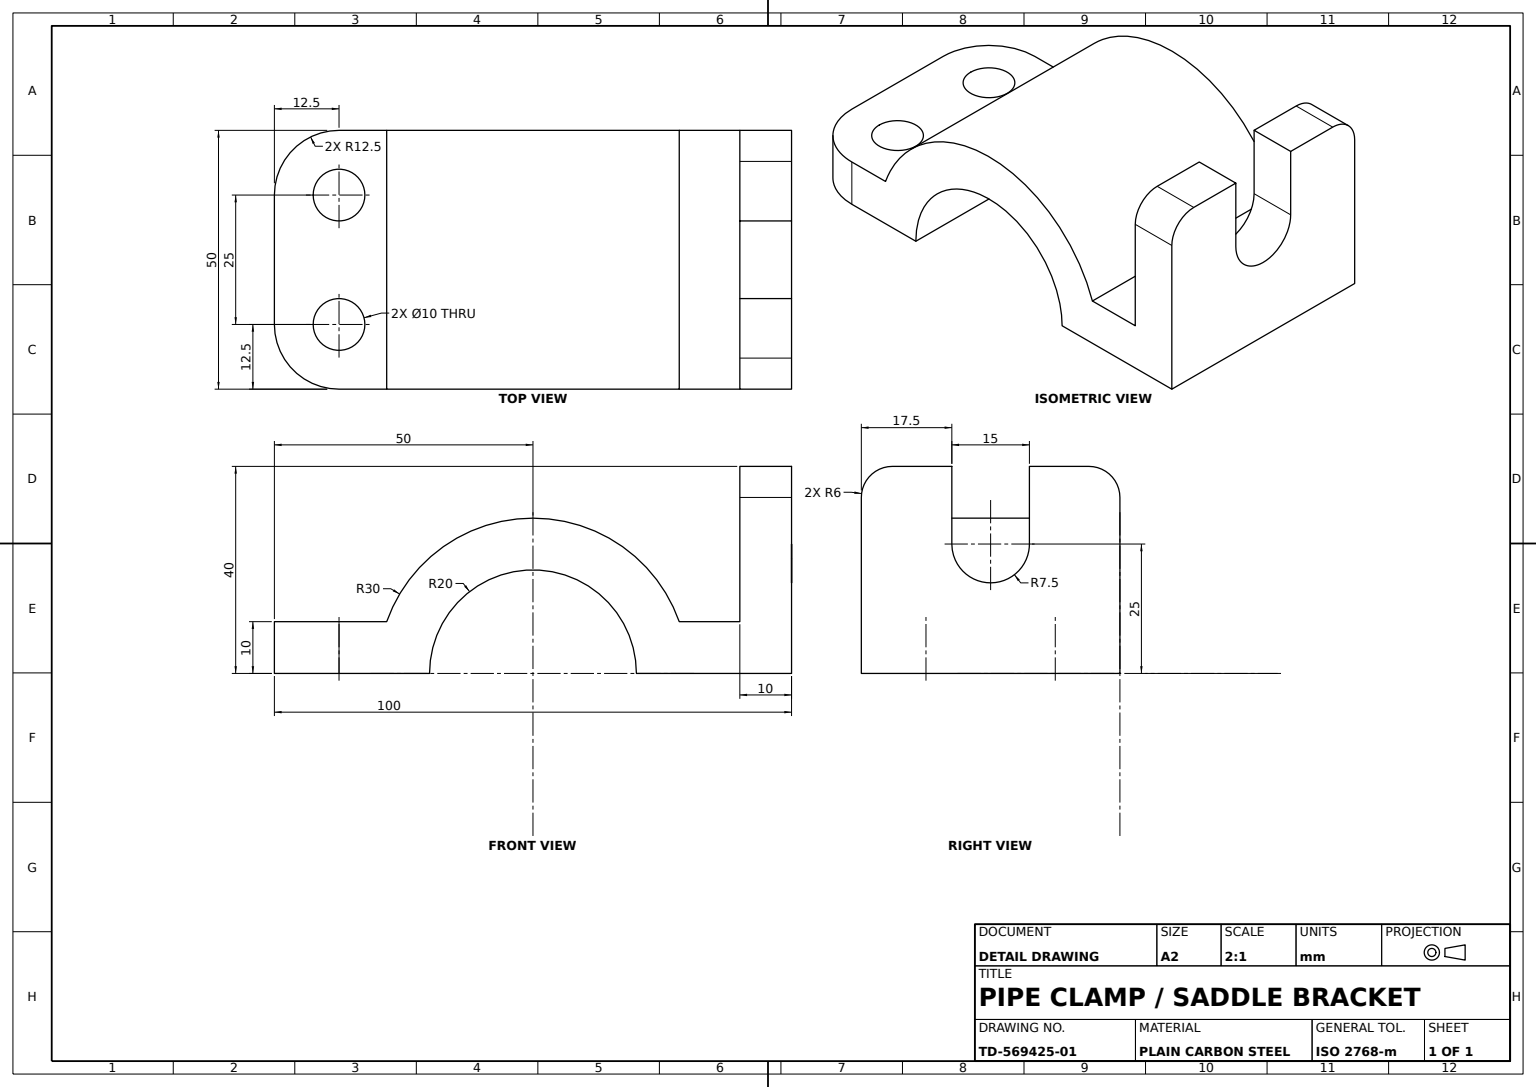
from build123d import *

# Parameters (mm, degrees)
BASE_BODY_EXTRUDE_DEPTH         = 25
FLANGE_END_ROUNDS_R12_5_R       = 12.5
EDGE_FILLETS_R6_R               = 6
FLANGE_BOLT_HOLES_2X_DEPTH      = 64.442887702
FLANGE_BOLT_HOLES_2X_DEPTH_BACK = 64.442887702
FLANGE_HOLES_SKETCH_R           = 5
FORK_SLOT_REACH                 = 112.567
FORK_SLOT_DIRECTION_2_DEPTH     = 111.566721937


with BuildPart() as part:
    # Base Profile Sketch → Base Body Extrude (new, symmetric)
    with BuildSketch(Plane.XY):
        with BuildLine():
            Line((50, 40), (50, 0))
            Line((50, 0), (20, 0))
            ThreePointArc((20, 0), (0, 20), (-20, 0))
            Line((-20, 0), (-50, 0))
            Line((-50, 0), (-50, 10))
            Line((-50, 10), (-28.284271247, 10))
            ThreePointArc((-28.284271247, 10), (0, 30), (28.284271247, 10))
            Line((28.284271247, 10), (40, 10))
            Line((40, 10), (40, 40))
            Line((40, 40), (50, 40))
        make_face()
    extrude(amount=BASE_BODY_EXTRUDE_DEPTH, both=True)

    # Flange End Rounds R12.5
    flange_end_rounds_r12_5_edges = [part.edges().sort_by_distance(p)[0] for p in [
        (-50, 5, 25),
        (-50, 5, -25),
    ]]
    fillet(flange_end_rounds_r12_5_edges, radius=FLANGE_END_ROUNDS_R12_5_R)

    # Edge Fillets R6
    edge_fillets_r6_edges = [part.edges().sort_by_distance(p)[0] for p in [
        (45, 40, -25),
        (45, 40, 25),
    ]]
    fillet(edge_fillets_r6_edges, radius=EDGE_FILLETS_R6_R)

    # Flange Holes Sketch → Flange Bolt Holes 2x (cut, two sides: drawn at the far end of the back side and taken through both)
    with BuildSketch(Plane(origin=(0, 10, 0), x_dir=(1, 0, 0), z_dir=(0, 1, 0)).offset(-FLANGE_BOLT_HOLES_2X_DEPTH_BACK)):
        with Locations(Location((-37.5, -12.5, 0), (0, 0, 180))):
            Circle(FLANGE_HOLES_SKETCH_R)
        with Locations(Location((-37.5, 12.5, 0), (0, 0, 180))):
            Circle(FLANGE_HOLES_SKETCH_R)
    extrude(amount=FLANGE_BOLT_HOLES_2X_DEPTH + FLANGE_BOLT_HOLES_2X_DEPTH_BACK, mode=Mode.SUBTRACT)

    # Fork Slot Sketch → Fork Slot (cut, up to next)
    with BuildSketch(Plane(origin=(50, 0, 0), x_dir=(0, 0, -1), z_dir=(1, 0, 0)), mode=Mode.PRIVATE) as fork_slot_sk1:
        with BuildLine():
            Line((7.5, 40), (7.5, 25))
            ThreePointArc((7.5, 25), (0, 17.5), (-7.5, 25))
            Line((-7.5, 25), (-7.5, 40))
            Line((-7.5, 40), (7.5, 40))
        make_face()
    fork_slot_tool1 = extrude(fork_slot_sk1.sketch, amount=-FORK_SLOT_REACH, mode=Mode.PRIVATE) & part.part
    add(fork_slot_tool1.solids().sort_by_distance((50, 29.487689, 0))[0], mode=Mode.SUBTRACT)

    # Fork Slot Sketch → Fork Slot direction 2 (cut)
    with BuildSketch(Plane(origin=(50, 0, 0), x_dir=(0, 0, -1), z_dir=(1, 0, 0))):
        with BuildLine():
            Line((7.5, 40), (7.5, 25))
            ThreePointArc((7.5, 25), (0, 17.5), (-7.5, 25))
            Line((-7.5, 25), (-7.5, 40))
            Line((-7.5, 40), (7.5, 40))
        make_face()
    extrude(amount=FORK_SLOT_DIRECTION_2_DEPTH, mode=Mode.SUBTRACT)


solid = part.part
